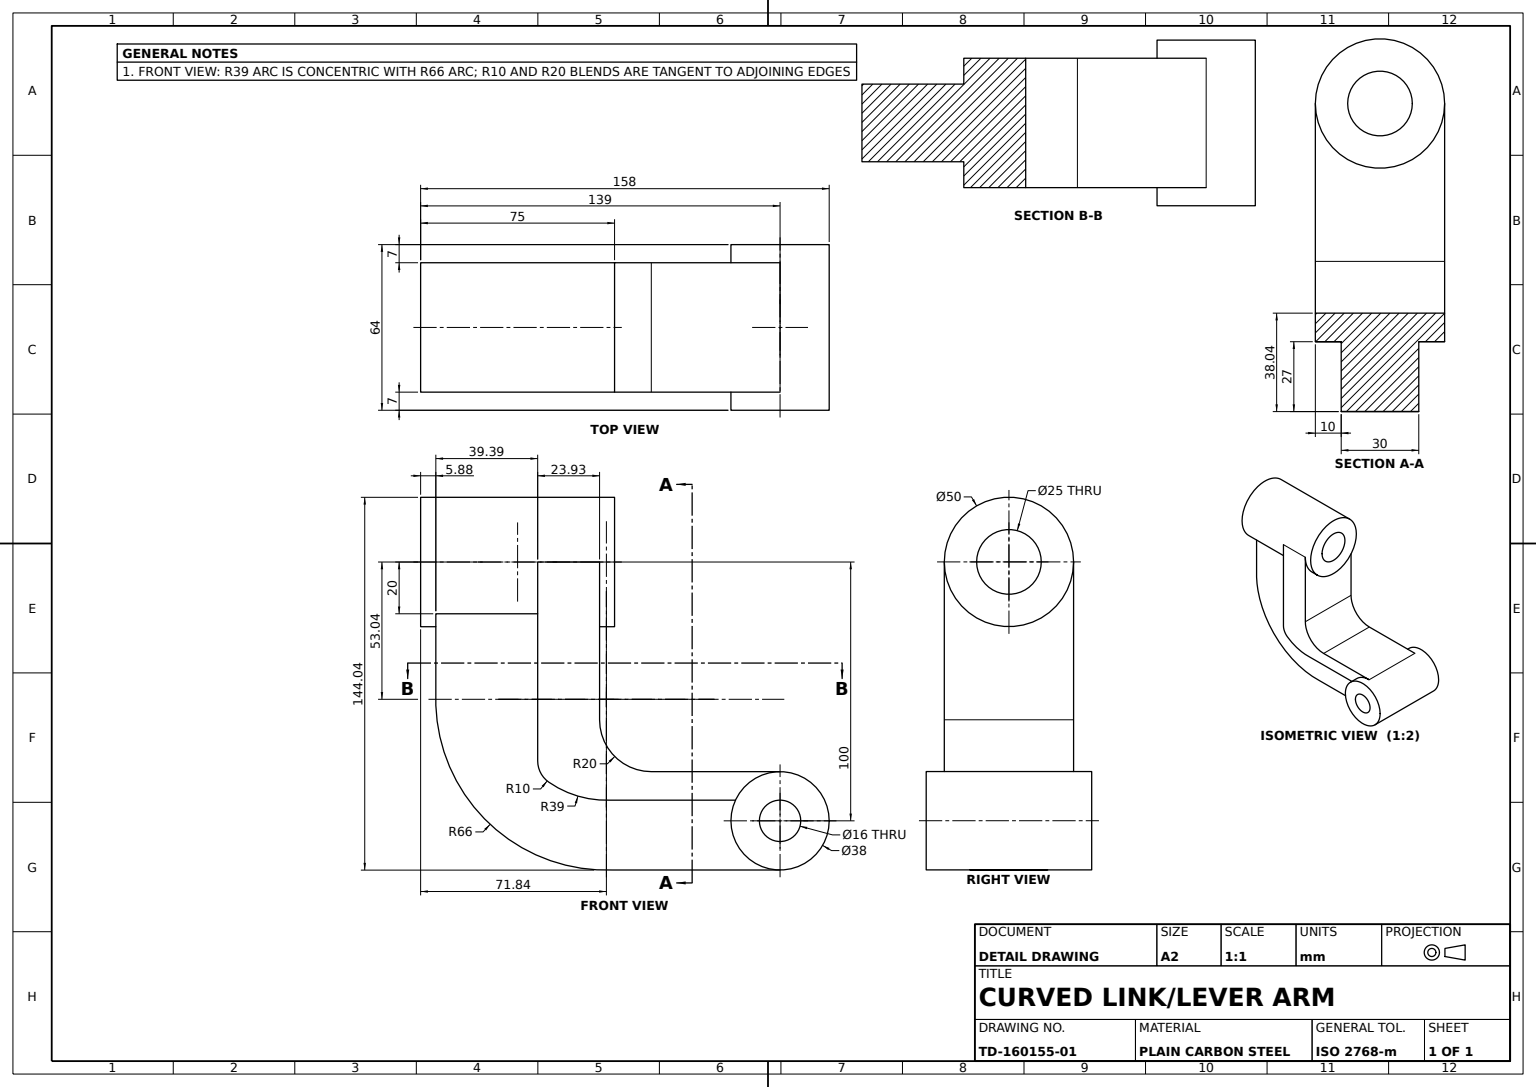
from build123d import *

# Parameters (mm, degrees)
HUB_1_PROFILE_R       = 25
HUB_1_BOSS_75MM_DEPTH = 37.5
HUB_2_PROFILE_R       = 19
HUB_2_BOSS_64MM_DEPTH = 32
CURVED_ARM_WEB_DEPTH  = 15
ARM_FLANGE_DEPTH      = 25
HUB_1_BORE_PROFILE_R  = 12.5
HUB_1_BORE_DEPTH      = 88
HUB_2_BORE_PROFILE_R  = 8
HUB_2_BORE_DEPTH      = 88


with BuildPart() as part:
    # Hub 1 Profile → Hub 1 Boss 75mm (new, symmetric)
    with BuildSketch(Plane(origin=(0, 0, 0), x_dir=(0, 0, -1), z_dir=(1, 0, 0))):
        Circle(HUB_1_PROFILE_R)
    extrude(amount=HUB_1_BOSS_75MM_DEPTH, both=True)



with BuildPart() as body_2:
    # Hub 2 Profile → Hub 2 Boss 64mm (new, symmetric)
    with BuildSketch(Plane.XY):
        with Locations((101.5, -100)):
            Circle(HUB_2_PROFILE_R)
    extrude(amount=HUB_2_BOSS_64MM_DEPTH, both=True)


with BuildPart() as part_1:
    add(part.part)

    add(body_2.part)  # Curved Arm Web merges body 2
    # Curved Arm Profile → Curved Arm Web (add, symmetric)
    with BuildSketch(Plane.XY):
        with BuildLine():
            Line((36.70784585, -119), (101.5, -119))
            ThreePointArc((101.5, -119), (85.489542295, -110.23060331), (84.258248254, -92.017394113))
            Line((84.258248254, -92.017394113), (35.73883627, -92.017394113))
            ThreePointArc((35.73883627, -92.017394113), (23.331450339, -90.456826651), (12.055799796, -85.049581394))
            ThreePointArc((12.055799796, -85.049581394), (8.905598759, -81.472069365), (7.769480814, -76.842642304))
            Line((7.769480814, -76.842642304), (7.769480814, -18.704046106))
            Line((7.769480814, -18.704046106), (-31.61832529, -18.704046106))
            Line((-31.61832529, -18.704046106), (-31.61832529, -25))
            Line((-31.61832529, -25), (-31.61832529, -55.411209028))
            ThreePointArc((-31.61832529, -55.411209028), (-10.624909538, -101.356417889), (36.70784585, -119))
        make_face()
    extrude(amount=CURVED_ARM_WEB_DEPTH, both=True)

    # Arm Flange Profile → Arm Flange (add, symmetric)
    with BuildSketch(Plane.XY):
        with BuildLine():
            Line((31.704445688, -20), (31.704445688, -61))
            ThreePointArc((31.704445688, -61), (37.562310065, -75.142135624), (51.704445688, -81))
            Line((51.704445688, -81), (101.5, -81))
            ThreePointArc((101.5, -81), (91.26939669, -83.989542295), (84.258248254, -92.017394113))
            Line((84.258248254, -92.017394113), (35.73883627, -92.017394113))
            ThreePointArc((35.73883627, -92.017394113), (23.331450339, -90.456826651), (12.055799796, -85.049581394))
            ThreePointArc((12.055799796, -85.049581394), (8.905598759, -81.472069365), (7.769480814, -76.842642304))
            Line((7.769480814, -76.842642304), (7.769480814, -20))
            Line((7.769480814, -20), (7.769480814, 0))
            Line((7.769480814, 0), (31.704445688, 0))
            Line((31.704445688, 0), (31.704445688, -20))
        make_face()
    extrude(amount=ARM_FLANGE_DEPTH, both=True)

    # Hub 1 Bore Profile → Hub 1 Bore (cut)
    with BuildSketch(Plane(origin=(37.5, 0, 0), x_dir=(0, 0, -1), z_dir=(1, 0, 0))):
        Circle(HUB_1_BORE_PROFILE_R)
    extrude(amount=-HUB_1_BORE_DEPTH, mode=Mode.SUBTRACT)

    # Hub 2 Bore Profile → Hub 2 Bore (cut)
    with BuildSketch(Plane(origin=(0, 0, -32), x_dir=(-1, 0, 0), z_dir=(0, 0, -1))):
        with Locations((-101.5, -100)):
            Circle(HUB_2_BORE_PROFILE_R)
    extrude(amount=-HUB_2_BORE_DEPTH, mode=Mode.SUBTRACT)


solid = part_1.part
